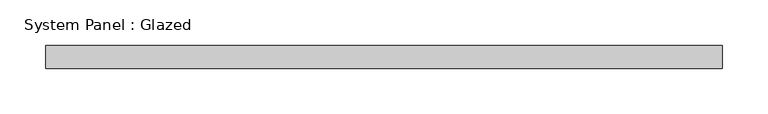
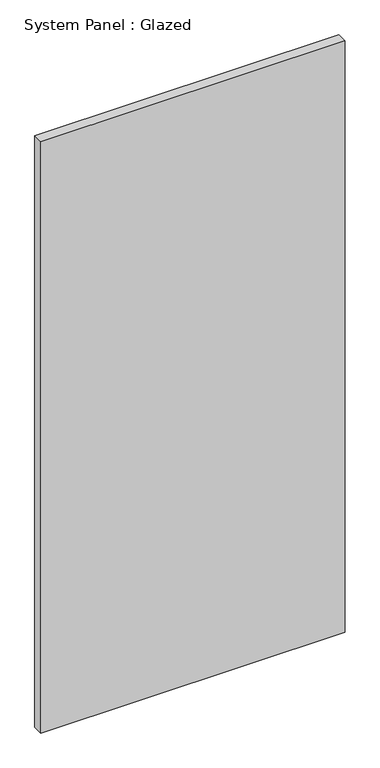
"""IFC4 building model written with IfcOpenShell, lengths in millimetres: plate geometry, System Panel : Glazed."""

from ifc_helpers import new_model, si_unit, origin, origin_with_axes, place, context, project, spatial, polyline, outline, extrude, source, transform, mapped, element, save


def system_panel_glazed_21f1ffe3(model_context):
    return source(origin(), model_context, "Body", "SweptSolid", [
        extrude(outline(polyline([(371.475, 19.05), (-371.475, 19.05), (-371.475, 44.45), (371.475, 44.45), (371.475, 19.05)])), origin_with_axes(), (0.0, 0.0, 1.0), 1526.9366569),
    ])


if __name__ == "__main__":
    model = new_model("IFC4")
    model_context = context("Model", 3, world=origin())
    ifc_project = project(units=[si_unit("LENGTHUNIT", "METRE", prefix="MILLI")], contexts=[model_context])
    site = spatial("IfcSite", under=ifc_project)
    building = spatial("IfcBuilding", under=site)
    placement = place(None, origin())
    system_panel_glazed_shape = system_panel_glazed_21f1ffe3(model_context)
    element("IfcPlate", 1, ObjectType="System Panel : Glazed", at=placement, inside=building, context=model_context, shape_type="MappedRepresentation", body=[
        mapped(system_panel_glazed_shape, transform((0.0, 0.0, 0.0), x_axis=(1.0, 0.0, 0.0), y_axis=(0.0, 1.0, 0.0), z_axis=(0.0, 0.0, 1.0))),
    ])
    save(model, "model.ifc")

# Revit data of these elements
# Type "System Panel : Glazed"
#   Construction Type Id = "GSP4R"
#   Analytic Construction = "1/8 in Pilkington single glazing"
#   Visual Light Transmittance = 0.9
#   Solar Heat Gain Coefficient = 0.86
#   Heat Transfer Coefficient (U) = 1.18115 BTU/(h·ft²·°F)
#   Define Thermal Properties by = 1
# Element 1 (IfcPlate, "System Panel : Glazed")
#   Materials on its faces: "Glass"
# Materials
#   "Glass": class "Glass", colour RGB 0 128 192, transparency 0.75, Description = "Soda Lime Glass", Cost = 0
